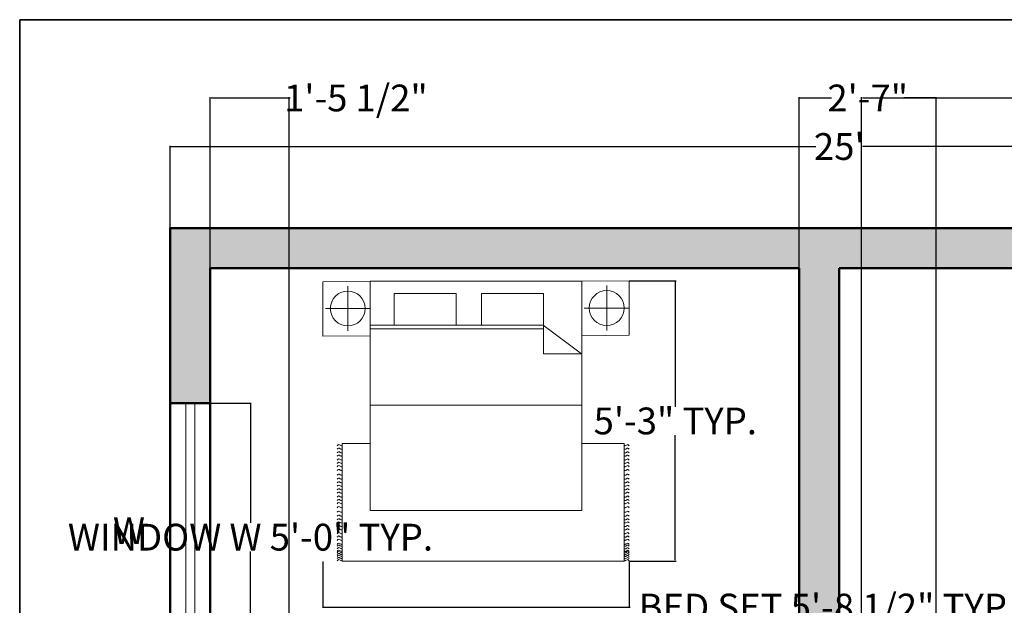
# Model space of a CAD drawing. Units: inches. Extents: x 125920 to 126336, y 366134 to 366735.
# Tile 5 of 6: x 125933 to 126153, y 366604 to 366735. Entities that reach past the tile are written whole.
import ezdxf

# ---------------------------------------------------------------- set-up
doc = ezdxf.new("R2010")
doc.units = ezdxf.units.IN
doc.header["$MEASUREMENT"] = 0
for name, color, linetype, lineweight in [('A-ANNO-DIMS', 2, 'Continuous', 18), ('A-ANNO-TEXT', 7, 'Continuous', 18), ('A-ANNO-TTLB', 7, 'Continuous', 35), ('A-FURN', 8, 'Continuous', 18), ('A-GLAZ', 4, 'Continuous', 18), ('A-WALL', 7, 'Continuous', 50)]:
    doc.layers.add(name, color=color, linetype=linetype, lineweight=lineweight)
doc.layers.add('A-WALL-PATT', color=18, linetype='Continuous', lineweight=13, true_color=0x000000)
doc.styles.get("Standard").update_dxf_attribs({"font": 'arial.ttf'})
doc.dimstyles.get("Standard").update_dxf_attribs({"dimtxt": 6, "dimasz": 0.18, "dimexe": 0.18, "dimexo": 0.0625, "dimgap": 0.09, "dimtad": 0, "dimtih": 1, "dimtoh": 1, "dimdec": 1, "dimzin": 0, "dimdsep": 46, "dimlunit": 3, "dimtxsty": 'Standard', "dimcen": 0.09, "dimadec": 0, "dimazin": 0, "dimtfac": 1, "dimtdec": 1, "dimtofl": 0, "dimtmove": 0, "dimatfit": 3, "dimfxl": 1, "dimtolj": 1, "dimtzin": 0, "dimarcsym": 0})

# ---------------------------------------------------------------- blocks, each defined once
blk = doc.blocks.new('*D3')
at = {"layer": 'A-ANNO-DIMS', "color": 0, "lineweight": -2, "transparency": 16777216}
for p, q in [((125966.47, 366688.86), (125966.47, 366707.25)), ((125966.65, 366707.07), (126111.24, 366707.07)), ((126266.29, 366707.07), (126121.71, 366707.07)), ((126266.47, 366688.86), (126266.47, 366707.25))]:
    blk.add_line(p, q, dxfattribs=at)
at = {"layer": 'A-ANNO-DIMS', "color": 0, "transparency": 16777216}
for points in [[(125966.65, 366707.1), (125966.65, 366707.04), (125966.47, 366707.07)], [(126266.29, 366707.1), (126266.29, 366707.04), (126266.47, 366707.07)]]:
    blk.add_solid(points, dxfattribs=at)
at = {"layer": 'Defpoints', "color": 0, "transparency": 16777216}
for p in [(126266.47, 366707.07), (125966.47, 366688.79), (126266.47, 366688.79)]:
    blk.add_point(p, dxfattribs=at)
at = {"layer": 'A-ANNO-DIMS', "color": 0, "transparency": 16777216, "insert": (126116.47, 366707.07), "char_height": 6, "attachment_point": 5}
blk.add_mtext("\\A1;25'", dxfattribs=at)
blk = doc.blocks.new('BED-DOUBLE-WITH-NIGHTSTANDS')
for p, q in [((5.6, 61.62), (5.6, 51.56)), ((63.65, 61.72), (63.65, 51.66)), ((10.63, 56.59), (0.57, 56.59)), ((68.68, 56.69), (58.62, 56.69)), ((49.39, 52.82), (10.63, 52.82)), ((49.44, 52), (10.63, 52)), ((49.39, 52.82), (58, 46.47)), ((49.44, 52.82), (49.44, 46.47)), ((49.44, 46.47), (58, 46.47)), ((58.05, 34.96), (10.63, 34.96)), ((4.36, 0), (4.36, 26.37)), ((4.36, 26.37), (10.65, 26.37)), ((58.05, 26.37), (67.59, 26.37)), ((67.59, 26.37), (67.59, 0)), ((67.59, 0), (4.36, 0))]:
    blk.add_line(p, q)
for points in [[(0, 50.39), (10.63, 50.5), (10.63, 62.68), (0, 62.58)], [(58.05, 62.68), (58.05, 11.37), (10.63, 11.37), (10.63, 62.68)], [(58.05, 50.5), (68.68, 50.6), (68.68, 62.78), (58.05, 62.68)], [(29.88, 59.98), (29.88, 52.82), (15.98, 52.82), (15.98, 59.98)], [(49.44, 59.98), (49.44, 52.82), (35.55, 52.82), (35.55, 59.98)]]:
    blk.add_lwpolyline(points, close=True)
for centre in [(5.6, 56.59), (63.65, 56.69)]:
    blk.add_circle(centre, 3.92)
for points, knots in [([(3.23, 25.84), (3.32, 25.96), (3.52, 26.2), (3.86, 25.96), (4.14, 25.78), (4.29, 25.89), (4.36, 25.94)], [0, 0, 0, 0, 0.400747, 0.791423, 1.067667, 1.29709, 1.29709, 1.29709, 1.29709]), ([(3.23, 25.06), (3.32, 25.18), (3.52, 25.42), (3.86, 25.18), (4.14, 25.01), (4.29, 25.11), (4.36, 25.16)], [0, 0, 0, 0, 0.400747, 0.791423, 1.067667, 1.29709, 1.29709, 1.29709, 1.29709]), ([(3.23, 24.24), (3.32, 24.36), (3.52, 24.6), (3.86, 24.36), (4.14, 24.19), (4.29, 24.3), (4.36, 24.34)], [0, 0, 0, 0, 0.400747, 0.791423, 1.067667, 1.29709, 1.29709, 1.29709, 1.29709]), ([(68.71, 25.84), (68.61, 25.96), (68.42, 26.2), (68.08, 25.96), (67.8, 25.78), (67.65, 25.89), (67.58, 25.94)], [0, 0, 0, 0, 0.400747, 0.791423, 1.067667, 1.29709, 1.29709, 1.29709, 1.29709]), ([(68.71, 25.06), (68.61, 25.18), (68.42, 25.42), (68.08, 25.18), (67.8, 25.01), (67.65, 25.11), (67.58, 25.16)], [0, 0, 0, 0, 0.400747, 0.791423, 1.067667, 1.29709, 1.29709, 1.29709, 1.29709]), ([(68.71, 24.24), (68.61, 24.36), (68.42, 24.6), (68.08, 24.36), (67.8, 24.19), (67.65, 24.3), (67.58, 24.34)], [0, 0, 0, 0, 0.400747, 0.791423, 1.067667, 1.29709, 1.29709, 1.29709, 1.29709]), ([(3.23, 23.51), (3.32, 23.63), (3.52, 23.87), (3.86, 23.63), (4.14, 23.46), (4.29, 23.57), (4.36, 23.62)], [0, 0, 0, 0, 0.400747, 0.791423, 1.067667, 1.29709, 1.29709, 1.29709, 1.29709]), ([(3.23, 22.63), (3.32, 22.75), (3.52, 22.99), (3.86, 22.75), (4.14, 22.58), (4.29, 22.69), (4.36, 22.73)], [0, 0, 0, 0, 0.400747, 0.791423, 1.067667, 1.29709, 1.29709, 1.29709, 1.29709]), ([(3.23, 21.88), (3.32, 22), (3.52, 22.24), (3.86, 22), (4.14, 21.83), (4.29, 21.93), (4.36, 21.98)], [0, 0, 0, 0, 0.400747, 0.791423, 1.067667, 1.29709, 1.29709, 1.29709, 1.29709]), ([(68.71, 23.51), (68.61, 23.63), (68.42, 23.87), (68.08, 23.63), (67.8, 23.46), (67.65, 23.57), (67.58, 23.62)], [0, 0, 0, 0, 0.400747, 0.791423, 1.067667, 1.29709, 1.29709, 1.29709, 1.29709]), ([(68.71, 22.63), (68.61, 22.75), (68.42, 22.99), (68.08, 22.75), (67.8, 22.58), (67.65, 22.69), (67.58, 22.73)], [0, 0, 0, 0, 0.400747, 0.791423, 1.067667, 1.29709, 1.29709, 1.29709, 1.29709]), ([(68.71, 21.88), (68.61, 22), (68.42, 22.24), (68.08, 22), (67.8, 21.83), (67.65, 21.93), (67.58, 21.98)], [0, 0, 0, 0, 0.400747, 0.791423, 1.067667, 1.29709, 1.29709, 1.29709, 1.29709]), ([(3.23, 21.15), (3.32, 21.27), (3.52, 21.51), (3.86, 21.27), (4.14, 21.1), (4.29, 21.21), (4.36, 21.25)], [0, 0, 0, 0, 0.400747, 0.791423, 1.067667, 1.29709, 1.29709, 1.29709, 1.29709]), ([(3.23, 20.27), (3.32, 20.39), (3.52, 20.63), (3.86, 20.39), (4.14, 20.22), (4.29, 20.32), (4.36, 20.37)], [0, 0, 0, 0, 0.400747, 0.791423, 1.067667, 1.29709, 1.29709, 1.29709, 1.29709]), ([(68.71, 21.15), (68.61, 21.27), (68.42, 21.51), (68.08, 21.27), (67.8, 21.1), (67.65, 21.21), (67.58, 21.25)], [0, 0, 0, 0, 0.400747, 0.791423, 1.067667, 1.29709, 1.29709, 1.29709, 1.29709]), ([(68.71, 20.27), (68.61, 20.39), (68.42, 20.63), (68.08, 20.39), (67.8, 20.22), (67.65, 20.32), (67.58, 20.37)], [0, 0, 0, 0, 0.400747, 0.791423, 1.067667, 1.29709, 1.29709, 1.29709, 1.29709]), ([(3.23, 19.23), (3.32, 19.35), (3.52, 19.59), (3.86, 19.35), (4.14, 19.18), (4.29, 19.29), (4.36, 19.33)], [0, 0, 0, 0, 0.400747, 0.791423, 1.067667, 1.29709, 1.29709, 1.29709, 1.29709]), ([(3.23, 18.35), (3.32, 18.47), (3.52, 18.71), (3.86, 18.47), (4.14, 18.3), (4.29, 18.4), (4.36, 18.45)], [0, 0, 0, 0, 0.400747, 0.791423, 1.067667, 1.29709, 1.29709, 1.29709, 1.29709]), ([(3.23, 17.53), (3.32, 17.65), (3.52, 17.89), (3.86, 17.65), (4.14, 17.48), (4.29, 17.59), (4.36, 17.64)], [0, 0, 0, 0, 0.400747, 0.791423, 1.067667, 1.29709, 1.29709, 1.29709, 1.29709]), ([(68.71, 19.23), (68.61, 19.35), (68.42, 19.59), (68.08, 19.35), (67.8, 19.18), (67.65, 19.29), (67.58, 19.33)], [0, 0, 0, 0, 0.400747, 0.791423, 1.067667, 1.29709, 1.29709, 1.29709, 1.29709]), ([(68.71, 18.35), (68.61, 18.47), (68.42, 18.71), (68.08, 18.47), (67.8, 18.3), (67.65, 18.4), (67.58, 18.45)], [0, 0, 0, 0, 0.400747, 0.791423, 1.067667, 1.29709, 1.29709, 1.29709, 1.29709]), ([(68.71, 17.53), (68.61, 17.65), (68.42, 17.89), (68.08, 17.65), (67.8, 17.48), (67.65, 17.59), (67.58, 17.64)], [0, 0, 0, 0, 0.400747, 0.791423, 1.067667, 1.29709, 1.29709, 1.29709, 1.29709]), ([(3.23, 16.76), (3.32, 16.88), (3.52, 17.12), (3.86, 16.88), (4.14, 16.7), (4.29, 16.81), (4.36, 16.86)], [0, 0, 0, 0, 0.400747, 0.791423, 1.067667, 1.29709, 1.29709, 1.29709, 1.29709]), ([(3.23, 15.94), (3.32, 16.06), (3.52, 16.3), (3.86, 16.06), (4.14, 15.89), (4.29, 16), (4.36, 16.04)], [0, 0, 0, 0, 0.400747, 0.791423, 1.067667, 1.29709, 1.29709, 1.29709, 1.29709]), ([(3.23, 15.21), (3.32, 15.33), (3.52, 15.57), (3.86, 15.33), (4.14, 15.16), (4.29, 15.27), (4.36, 15.32)], [0, 0, 0, 0, 0.400747, 0.791423, 1.067667, 1.29709, 1.29709, 1.29709, 1.29709]), ([(68.71, 16.76), (68.61, 16.88), (68.42, 17.12), (68.08, 16.88), (67.8, 16.7), (67.65, 16.81), (67.58, 16.86)], [0, 0, 0, 0, 0.400747, 0.791423, 1.067667, 1.29709, 1.29709, 1.29709, 1.29709]), ([(68.71, 15.94), (68.61, 16.06), (68.42, 16.3), (68.08, 16.06), (67.8, 15.89), (67.65, 16), (67.58, 16.04)], [0, 0, 0, 0, 0.400747, 0.791423, 1.067667, 1.29709, 1.29709, 1.29709, 1.29709]), ([(68.71, 15.21), (68.61, 15.33), (68.42, 15.57), (68.08, 15.33), (67.8, 15.16), (67.65, 15.27), (67.58, 15.32)], [0, 0, 0, 0, 0.400747, 0.791423, 1.067667, 1.29709, 1.29709, 1.29709, 1.29709]), ([(3.23, 14.33), (3.32, 14.45), (3.52, 14.69), (3.86, 14.45), (4.14, 14.28), (4.29, 14.38), (4.36, 14.43)], [0, 0, 0, 0, 0.400747, 0.791423, 1.067667, 1.29709, 1.29709, 1.29709, 1.29709]), ([(3.23, 13.58), (3.32, 13.7), (3.52, 13.94), (3.86, 13.7), (4.14, 13.53), (4.29, 13.63), (4.36, 13.68)], [0, 0, 0, 0, 0.400747, 0.791423, 1.067667, 1.29709, 1.29709, 1.29709, 1.29709]), ([(68.71, 14.33), (68.61, 14.45), (68.42, 14.69), (68.08, 14.45), (67.8, 14.28), (67.65, 14.38), (67.58, 14.43)], [0, 0, 0, 0, 0.400747, 0.791423, 1.067667, 1.29709, 1.29709, 1.29709, 1.29709]), ([(68.71, 13.58), (68.61, 13.7), (68.42, 13.94), (68.08, 13.7), (67.8, 13.53), (67.65, 13.63), (67.58, 13.68)], [0, 0, 0, 0, 0.400747, 0.791423, 1.067667, 1.29709, 1.29709, 1.29709, 1.29709]), ([(3.23, 12.85), (3.32, 12.97), (3.52, 13.21), (3.86, 12.97), (4.14, 12.8), (4.29, 12.9), (4.36, 12.95)], [0, 0, 0, 0, 0.400747, 0.791423, 1.067667, 1.29709, 1.29709, 1.29709, 1.29709]), ([(3.23, 11.97), (3.32, 12.09), (3.52, 12.33), (3.86, 12.09), (4.14, 11.92), (4.29, 12.02), (4.36, 12.07)], [0, 0, 0, 0, 0.400747, 0.791423, 1.067667, 1.29709, 1.29709, 1.29709, 1.29709]), ([(3.23, 10.93), (3.32, 11.05), (3.52, 11.29), (3.86, 11.05), (4.14, 10.88), (4.29, 10.99), (4.36, 11.03)], [0, 0, 0, 0, 0.400747, 0.791423, 1.067667, 1.29709, 1.29709, 1.29709, 1.29709]), ([(68.71, 12.85), (68.61, 12.97), (68.42, 13.21), (68.08, 12.97), (67.8, 12.8), (67.65, 12.9), (67.58, 12.95)], [0, 0, 0, 0, 0.400747, 0.791423, 1.067667, 1.29709, 1.29709, 1.29709, 1.29709]), ([(68.71, 11.97), (68.61, 12.09), (68.42, 12.33), (68.08, 12.09), (67.8, 11.92), (67.65, 12.02), (67.58, 12.07)], [0, 0, 0, 0, 0.400747, 0.791423, 1.067667, 1.29709, 1.29709, 1.29709, 1.29709]), ([(68.71, 10.93), (68.61, 11.05), (68.42, 11.29), (68.08, 11.05), (67.8, 10.88), (67.65, 10.99), (67.58, 11.03)], [0, 0, 0, 0, 0.400747, 0.791423, 1.067667, 1.29709, 1.29709, 1.29709, 1.29709]), ([(3.23, 10.05), (3.32, 10.17), (3.52, 10.41), (3.86, 10.17), (4.14, 10), (4.29, 10.1), (4.36, 10.15)], [0, 0, 0, 0, 0.400747, 0.791423, 1.067667, 1.29709, 1.29709, 1.29709, 1.29709]), ([(3.23, 9.23), (3.32, 9.35), (3.52, 9.59), (3.86, 9.35), (4.14, 9.18), (4.29, 9.29), (4.36, 9.34)], [0, 0, 0, 0, 0.400747, 0.791423, 1.067667, 1.29709, 1.29709, 1.29709, 1.29709]), ([(68.71, 10.05), (68.61, 10.17), (68.42, 10.41), (68.08, 10.17), (67.8, 10), (67.65, 10.1), (67.58, 10.15)], [0, 0, 0, 0, 0.400747, 0.791423, 1.067667, 1.29709, 1.29709, 1.29709, 1.29709]), ([(68.71, 9.23), (68.61, 9.35), (68.42, 9.59), (68.08, 9.35), (67.8, 9.18), (67.65, 9.29), (67.58, 9.34)], [0, 0, 0, 0, 0.400747, 0.791423, 1.067667, 1.29709, 1.29709, 1.29709, 1.29709]), ([(3.23, 8.54), (3.32, 8.66), (3.52, 8.9), (3.86, 8.66), (4.14, 8.49), (4.29, 8.6), (4.36, 8.65)], [0, 0, 0, 0, 0.400747, 0.791423, 1.067667, 1.29709, 1.29709, 1.29709, 1.29709]), ([(3.23, 7.73), (3.32, 7.85), (3.52, 8.09), (3.86, 7.85), (4.14, 7.68), (4.29, 7.78), (4.36, 7.83)], [0, 0, 0, 0, 0.400747, 0.791423, 1.067667, 1.29709, 1.29709, 1.29709, 1.29709]), ([(3.23, 7), (3.32, 7.12), (3.52, 7.36), (3.86, 7.12), (4.14, 6.95), (4.29, 7.05), (4.36, 7.1)], [0, 0, 0, 0, 0.400747, 0.791423, 1.067667, 1.29709, 1.29709, 1.29709, 1.29709]), ([(68.71, 8.54), (68.61, 8.66), (68.42, 8.9), (68.08, 8.66), (67.8, 8.49), (67.65, 8.6), (67.58, 8.65)], [0, 0, 0, 0, 0.400747, 0.791423, 1.067667, 1.29709, 1.29709, 1.29709, 1.29709]), ([(68.71, 7.73), (68.61, 7.85), (68.42, 8.09), (68.08, 7.85), (67.8, 7.68), (67.65, 7.78), (67.58, 7.83)], [0, 0, 0, 0, 0.400747, 0.791423, 1.067667, 1.29709, 1.29709, 1.29709, 1.29709]), ([(68.71, 7), (68.61, 7.12), (68.42, 7.36), (68.08, 7.12), (67.8, 6.95), (67.65, 7.05), (67.58, 7.1)], [0, 0, 0, 0, 0.400747, 0.791423, 1.067667, 1.29709, 1.29709, 1.29709, 1.29709]), ([(3.23, 6.12), (3.32, 6.24), (3.52, 6.48), (3.86, 6.24), (4.14, 6.07), (4.29, 6.17), (4.36, 6.22)], [0, 0, 0, 0, 0.400747, 0.791423, 1.067667, 1.29709, 1.29709, 1.29709, 1.29709]), ([(3.23, 5.36), (3.32, 5.49), (3.52, 5.73), (3.86, 5.49), (4.14, 5.31), (4.29, 5.42), (4.36, 5.47)], [0, 0, 0, 0, 0.400747, 0.791423, 1.067667, 1.29709, 1.29709, 1.29709, 1.29709]), ([(3.23, 4.64), (3.32, 4.76), (3.52, 5), (3.86, 4.76), (4.14, 4.59), (4.29, 4.69), (4.36, 4.74)], [0, 0, 0, 0, 0.400747, 0.791423, 1.067667, 1.29709, 1.29709, 1.29709, 1.29709]), ([(68.71, 6.12), (68.61, 6.24), (68.42, 6.48), (68.08, 6.24), (67.8, 6.07), (67.65, 6.17), (67.58, 6.22)], [0, 0, 0, 0, 0.400747, 0.791423, 1.067667, 1.29709, 1.29709, 1.29709, 1.29709]), ([(68.71, 5.36), (68.61, 5.49), (68.42, 5.73), (68.08, 5.49), (67.8, 5.31), (67.65, 5.42), (67.58, 5.47)], [0, 0, 0, 0, 0.400747, 0.791423, 1.067667, 1.29709, 1.29709, 1.29709, 1.29709]), ([(68.71, 4.64), (68.61, 4.76), (68.42, 5), (68.08, 4.76), (67.8, 4.59), (67.66, 4.69), (67.59, 4.73)], [0, 0, 0, 0, 0.400747, 0.791423, 1.067667, 1.283686, 1.283686, 1.283686, 1.283686]), ([(3.23, 3.75), (3.32, 3.88), (3.52, 4.12), (3.86, 3.88), (4.14, 3.7), (4.29, 3.81), (4.36, 3.86)], [0, 0, 0, 0, 0.400747, 0.791423, 1.067667, 1.29709, 1.29709, 1.29709, 1.29709]), ([(3.23, 3.33), (3.32, 3.45), (3.52, 3.7), (3.86, 3.44), (4.14, 3.27), (4.29, 3.38), (4.36, 3.43)], [0, 0, 0, 0, 0.407265, 0.802015, 1.07826, 1.307683, 1.307683, 1.307683, 1.307683]), ([(3.23, 2.76), (3.32, 2.88), (3.52, 3.12), (3.86, 2.88), (4.14, 2.71), (4.29, 2.81), (4.36, 2.86)], [0, 0, 0, 0, 0.400747, 0.791423, 1.067667, 1.29709, 1.29709, 1.29709, 1.29709]), ([(3.23, 2.18), (3.32, 2.31), (3.52, 2.55), (3.86, 2.31), (4.14, 2.13), (4.29, 2.24), (4.36, 2.29)], [0, 0, 0, 0, 0.400747, 0.791423, 1.067667, 1.29709, 1.29709, 1.29709, 1.29709]), ([(68.71, 3.75), (68.61, 3.88), (68.42, 4.11), (68.08, 3.88), (67.8, 3.7), (67.66, 3.81), (67.59, 3.85)], [0, 0, 0, 0, 0.400747, 0.791423, 1.067667, 1.283686, 1.283686, 1.283686, 1.283686]), ([(68.71, 3.33), (68.61, 3.45), (68.42, 3.69), (68.08, 3.45), (67.8, 3.27), (67.66, 3.38), (67.59, 3.42)], [0, 0, 0, 0, 0.402903, 0.794912, 1.071156, 1.287177, 1.287177, 1.287177, 1.287177]), ([(68.71, 2.73), (68.61, 2.85), (68.42, 3.09), (68.08, 2.85), (67.8, 2.68), (67.66, 2.78), (67.59, 2.82)], [0, 0, 0, 0, 0.400747, 0.791423, 1.067667, 1.283686, 1.283686, 1.283686, 1.283686]), ([(68.71, 2.16), (68.61, 2.28), (68.42, 2.52), (68.08, 2.28), (67.8, 2.11), (67.66, 2.21), (67.59, 2.25)], [0, 0, 0, 0, 0.400747, 0.791423, 1.067667, 1.283686, 1.283686, 1.283686, 1.283686]), ([(3.23, 1.88), (3.32, 2), (3.52, 2.24), (3.86, 2), (4.14, 1.82), (4.29, 1.93), (4.36, 1.98)], [0, 0, 0, 0, 0.400747, 0.791423, 1.067667, 1.29709, 1.29709, 1.29709, 1.29709]), ([(3.23, 1.46), (3.32, 1.58), (3.52, 1.82), (3.86, 1.58), (4.14, 1.41), (4.29, 1.51), (4.36, 1.56)], [0, 0, 0, 0, 0.400747, 0.791423, 1.067667, 1.29709, 1.29709, 1.29709, 1.29709]), ([(3.23, 1.06), (3.32, 1.18), (3.52, 1.42), (3.86, 1.18), (4.14, 1.01), (4.29, 1.11), (4.36, 1.16)], [0, 0, 0, 0, 0.400747, 0.791423, 1.067667, 1.29709, 1.29709, 1.29709, 1.29709]), ([(3.23, 0.57), (3.32, 0.7), (3.52, 0.94), (3.86, 0.7), (4.14, 0.52), (4.29, 0.63), (4.36, 0.68)], [0, 0, 0, 0, 0.400747, 0.791423, 1.067667, 1.29709, 1.29709, 1.29709, 1.29709]), ([(3.23, 0.07), (3.32, 0.19), (3.52, 0.43), (3.86, 0.19), (4.14, 0.02), (4.29, 0.13), (4.36, 0.18)], [0, 0, 0, 0, 0.400747, 0.791423, 1.067667, 1.29709, 1.29709, 1.29709, 1.29709]), ([(68.71, 1.43), (68.61, 1.55), (68.42, 1.79), (68.08, 1.55), (67.8, 1.38), (67.65, 1.48), (67.58, 1.53)], [0, 0, 0, 0, 0.400747, 0.791423, 1.067667, 1.29709, 1.29709, 1.29709, 1.29709]), ([(68.71, 1.03), (68.61, 1.15), (68.42, 1.39), (68.08, 1.15), (67.8, 0.98), (67.65, 1.09), (67.58, 1.13)], [0, 0, 0, 0, 0.400747, 0.791423, 1.067667, 1.29709, 1.29709, 1.29709, 1.29709]), ([(68.71, 0.55), (68.61, 0.67), (68.42, 0.91), (68.08, 0.67), (67.8, 0.49), (67.65, 0.6), (67.58, 0.65)], [0, 0, 0, 0, 0.400747, 0.791423, 1.067667, 1.29709, 1.29709, 1.29709, 1.29709]), ([(68.71, 0.07), (68.61, 0.19), (68.42, 0.43), (68.08, 0.19), (67.8, 0.02), (67.65, 0.13), (67.58, 0.18)], [0, 0, 0, 0, 0.400747, 0.791423, 1.067667, 1.29709, 1.29709, 1.29709, 1.29709]), ([(68.71, 1.85), (68.61, 1.97), (68.42, 2.21), (68.08, 1.97), (67.8, 1.8), (67.66, 1.9), (67.59, 1.94)], [0, 0, 0, 0, 0.400747, 0.791423, 1.067667, 1.283686, 1.283686, 1.283686, 1.283686])]:
    blk.add_open_spline(points, degree=3, knots=knots)
blk = doc.blocks.new('WIN-60')
for p, q in [((0, 0), (0, 60)), ((3.5, 0), (3.5, 60)), ((5.5, 60), (5.5, 0)), ((9, 60), (9, 0))]:
    blk.add_line(p, q)
blk = doc.blocks.new('*D13')
at = {"layer": 'A-ANNO-DIMS', "color": 0, "lineweight": -2, "transparency": 16777216}
for p, q in [((125975.54, 366649.55), (125984.65, 366649.55)), ((125984.47, 366649.37), (125984.47, 366622.75)), ((125984.47, 366589.73), (125984.47, 366616.36)), ((125975.54, 366589.55), (125984.65, 366589.55))]:
    blk.add_line(p, q, dxfattribs=at)
at = {"layer": 'A-ANNO-DIMS', "color": 0, "transparency": 16777216}
for points in [[(125984.44, 366649.37), (125984.5, 366649.37), (125984.47, 366649.55)], [(125984.44, 366589.73), (125984.5, 366589.73), (125984.47, 366589.55)]]:
    blk.add_solid(points, dxfattribs=at)
at = {"layer": 'Defpoints', "color": 0, "transparency": 16777216}
for p in [(125975.47, 366649.55), (125984.47, 366649.55), (125975.47, 366589.55)]:
    blk.add_point(p, dxfattribs=at)
at = {"layer": 'A-ANNO-DIMS', "color": 0, "transparency": 16777216, "insert": (125984.47, 366619.55), "char_height": 6, "attachment_point": 5}
blk.add_mtext('\\A1;WINDOW W 5\'-0" TYP.', dxfattribs=at)
blk = doc.blocks.new('*D19')
at = {"layer": 'A-ANNO-DIMS', "color": 0, "lineweight": -2, "transparency": 16777216}
for p, q in [((126000.69, 366614.13), (126000.69, 366603.71)), ((126069.4, 366614.13), (126069.4, 366603.71)), ((126000.87, 366603.89), (126069.22, 366603.89)), ((126069.4, 366603.89), (126069.58, 366603.89))]:
    blk.add_line(p, q, dxfattribs=at)
at = {"layer": 'A-ANNO-DIMS', "color": 0, "transparency": 16777216}
for points in [[(126000.87, 366603.92), (126000.87, 366603.86), (126000.69, 366603.89)], [(126069.22, 366603.92), (126069.22, 366603.86), (126069.4, 366603.89)]]:
    blk.add_solid(points, dxfattribs=at)
at = {"layer": 'Defpoints', "color": 0, "transparency": 16777216}
for p in [(126000.69, 366614.19), (126069.4, 366614.19), (126069.4, 366603.89)]:
    blk.add_point(p, dxfattribs=at)
at = {"layer": 'A-ANNO-DIMS', "color": 0, "transparency": 16777216, "insert": (126113.91, 366603.89), "char_height": 6, "attachment_point": 5}
blk.add_mtext('\\A1;BED SET 5\'-8 1/2" TYP.', dxfattribs=at)
blk = doc.blocks.new('*D20')
at = {"layer": 'A-ANNO-DIMS', "color": 0, "lineweight": -2, "transparency": 16777216}
for p, q in [((126069.46, 366676.98), (126079.89, 366676.98)), ((126079.71, 366676.8), (126079.71, 366648.74)), ((126079.71, 366614.37), (126079.71, 366642.43)), ((126069.46, 366614.19), (126079.89, 366614.19))]:
    blk.add_line(p, q, dxfattribs=at)
at = {"layer": 'A-ANNO-DIMS', "color": 0, "transparency": 16777216}
for points in [[(126079.68, 366676.8), (126079.74, 366676.8), (126079.71, 366676.98)], [(126079.68, 366614.37), (126079.74, 366614.37), (126079.71, 366614.19)]]:
    blk.add_solid(points, dxfattribs=at)
at = {"layer": 'Defpoints', "color": 0, "transparency": 16777216}
for p in [(126069.4, 366676.98), (126079.71, 366676.98), (126069.4, 366614.19)]:
    blk.add_point(p, dxfattribs=at)
at = {"layer": 'A-ANNO-DIMS', "color": 0, "transparency": 16777216, "insert": (126079.71, 366645.59), "char_height": 6, "attachment_point": 5}
blk.add_mtext('\\A1;5\'-3" TYP.', dxfattribs=at)
blk = doc.blocks.new('*D40')
at = {"layer": 'A-ANNO-DIMS', "color": 0, "lineweight": -2, "transparency": 16777216}
for p, q in [((126107.47, 366288.86), (126107.47, 366718.12)), ((126107.65, 366717.94), (126114.73, 366717.94)), ((126138.05, 366717.94), (126130.97, 366717.94)), ((126138.23, 366288.86), (126138.23, 366718.12))]:
    blk.add_line(p, q, dxfattribs=at)
at = {"layer": 'A-ANNO-DIMS', "color": 0, "transparency": 16777216}
for points in [[(126107.65, 366717.97), (126107.65, 366717.91), (126107.47, 366717.94)], [(126138.05, 366717.97), (126138.05, 366717.91), (126138.23, 366717.94)]]:
    blk.add_solid(points, dxfattribs=at)
at = {"layer": 'Defpoints', "color": 0, "transparency": 16777216}
for p in [(126138.23, 366717.94), (126107.47, 366288.79), (126138.23, 366288.79)]:
    blk.add_point(p, dxfattribs=at)
at = {"layer": 'A-ANNO-DIMS', "color": 0, "transparency": 16777216, "insert": (126122.85, 366717.94), "char_height": 6, "attachment_point": 5}
blk.add_mtext('\\A1;2\'-7"', dxfattribs=at)
blk = doc.blocks.new('*D41')
at = {"layer": 'A-ANNO-DIMS', "color": 0, "lineweight": -2, "transparency": 16777216}
for p, q in [((126121.47, 366216.86), (126121.47, 366718.12)), ((126121.65, 366717.94), (126163.4, 366717.94)), ((126221.29, 366717.94), (126179.54, 366717.94)), ((126221.47, 366216.86), (126221.47, 366718.12))]:
    blk.add_line(p, q, dxfattribs=at)
at = {"layer": 'A-ANNO-DIMS', "color": 0, "transparency": 16777216}
for points in [[(126121.65, 366717.97), (126121.65, 366717.91), (126121.47, 366717.94)], [(126221.29, 366717.97), (126221.29, 366717.91), (126221.47, 366717.94)]]:
    blk.add_solid(points, dxfattribs=at)
at = {"layer": 'Defpoints', "color": 0, "transparency": 16777216}
for p in [(126221.47, 366717.94), (126121.47, 366216.79), (126221.47, 366216.79)]:
    blk.add_point(p, dxfattribs=at)
at = {"layer": 'A-ANNO-DIMS', "color": 0, "transparency": 16777216, "insert": (126171.47, 366717.94), "char_height": 6, "attachment_point": 5}
blk.add_mtext('\\A1;8\'-4"', dxfattribs=at)
blk = doc.blocks.new('*D45')
at = {"layer": 'A-ANNO-DIMS', "color": 0, "lineweight": -2, "transparency": 16777216}
for p, q in [((125975.47, 366216.86), (125975.47, 366718.12)), ((125975.65, 366717.94), (125992.98, 366717.94)), ((125993.16, 366235.36), (125993.16, 366718.12)), ((125993.16, 366717.94), (125993.34, 366717.94))]:
    blk.add_line(p, q, dxfattribs=at)
at = {"layer": 'A-ANNO-DIMS', "color": 0, "transparency": 16777216}
for points in [[(125975.65, 366717.97), (125975.65, 366717.91), (125975.47, 366717.94)], [(125992.98, 366717.97), (125992.98, 366717.91), (125993.16, 366717.94)]]:
    blk.add_solid(points, dxfattribs=at)
at = {"layer": 'Defpoints', "color": 0, "transparency": 16777216}
for p in [(125993.16, 366717.94), (125993.16, 366235.3), (125975.47, 366216.79)]:
    blk.add_point(p, dxfattribs=at)
at = {"layer": 'A-ANNO-DIMS', "color": 0, "transparency": 16777216, "insert": (126008.11, 366717.94), "char_height": 6, "attachment_point": 5}
blk.add_mtext('\\A1;1\'-5 1/2"', dxfattribs=at)

msp = doc.modelspace()

# ---------------------------------------------------------------- hatches: boundary and pattern name
at = {"layer": 'A-WALL-PATT'}
h = msp.add_hatch(color=256, dxfattribs=at)
h.dxf.hatch_style = 1
h.paths.add_polyline_path([(126266.47, 366688.79), (125966.47, 366688.79), (125966.47, 366649.55), (125975.47, 366649.55), (125975.47, 366679.79), (126107.47, 366679.79), (126107.47, 366547.79), (126106.47, 366547.79), (126106.47, 366538.79), (126107.47, 366538.79), (126117.47, 366538.79), (126117.47, 366547.79), (126116.47, 366547.79), (126116.47, 366679.79), (126257.47, 366679.79), (126257.47, 366648.33), (126266.47, 366648.33)])
h.paths.add_polyline_path([(126070.47, 366547.79), (125975.47, 366547.79), (125975.47, 366589.55), (125966.47, 366589.55), (125966.47, 366528.42), (125975.47, 366528.42), (125975.47, 366538.79), (126059.47, 366538.79), (126059.47, 366515.79), (126063.97, 366515.79), (126063.97, 366538.79), (126070.47, 366538.79)])
h.paths.add_polyline_path([(125975.47, 366486.29), (126063.97, 366486.29), (126063.97, 366491.79), (126059.47, 366491.79), (126059.47, 366490.79), (125975.47, 366490.79), (125975.47, 366504.42), (125966.47, 366504.42), (125966.47, 366437.07), (125975.47, 366437.07)])
h.paths.add_polyline_path([(125975.47, 366312.79), (126022.47, 366312.79), (126022.47, 366317.29), (125975.47, 366317.29), (125975.47, 366377.07), (125966.47, 366377.07), (125966.47, 366207.79), (125987.64, 366207.79), (125987.64, 366216.79), (125975.47, 366216.79)])
h.paths.add_polyline_path([(126063.97, 366216.79), (126063.97, 366312.79), (126070.47, 366312.79), (126070.47, 366317.29), (126058.47, 366317.29), (126058.47, 366312.79), (126059.47, 366312.79), (126059.47, 366216.79), (126047.64, 366216.79), (126047.64, 366207.79), (126063.97, 366207.79)])
h.paths.add_polyline_path([(126221.47, 366216.79), (126116.47, 366216.79), (126107.47, 366216.79), (126107.47, 366207.79), (126221.47, 366207.79)])
h.paths.add_polyline_path([(126266.47, 366336.48), (126257.47, 366336.48), (126257.47, 366297.79), (126174.23, 366297.79), (126174.23, 366288.79), (126257.47, 366288.79), (126257.47, 366207.79), (126266.47, 366207.79)])
h.paths.add_polyline_path([(126138.23, 366297.79), (126116.47, 366297.79), (126116.47, 366433.79), (126117.47, 366433.79), (126117.47, 366438.29), (126116.47, 366438.29), (126107.47, 366438.29), (126107.47, 366317.29), (126106.47, 366317.29), (126106.47, 366312.79), (126107.47, 366312.79), (126107.47, 366288.79), (126116.47, 366288.79), (126138.23, 366288.79)])
h.paths.add_polyline_path([(126266.47, 366449.1), (126257.47, 366449.1), (126257.47, 366438.29), (126256.47, 366438.29), (126256.47, 366433.79), (126257.47, 366433.79), (126257.47, 366396.48), (126266.47, 366396.48)])
h.paths.add_polyline_path([(126232.47, 366438.29), (126180.47, 366438.29), (126180.47, 366486.29), (126257.47, 366486.29), (126257.47, 366473.1), (126266.47, 366473.1), (126266.47, 366504.78), (126257.47, 366504.78), (126257.47, 366490.79), (126180.47, 366490.79), (126180.47, 366538.79), (126232.47, 366538.79), (126232.47, 366547.79), (126153.47, 366547.79), (126153.47, 366538.79), (126175.97, 366538.79), (126175.97, 366438.29), (126153.47, 366438.29), (126153.47, 366433.79), (126232.47, 366433.79)])
h.paths.add_polyline_path([(126266.47, 366588.33), (126257.47, 366588.33), (126257.47, 366547.79), (126256.47, 366547.79), (126256.47, 366538.79), (126257.47, 366538.79), (126257.47, 366528.78), (126266.47, 366528.78)])

# ---------------------------------------------------------------- linework, layer by layer
at = {"layer": 'A-ANNO-TTLB'}
msp.add_lwpolyline([(125932.73, 366735.48), (126336.24, 366735.48), (126336.24, 366133.52), (125932.73, 366133.52)], close=True, dxfattribs=at)
at = {"layer": 'A-WALL'}
for p, q in [((125966.47, 366688.79), (126266.47, 366688.79)), ((125966.47, 366688.79), (125966.47, 366207.79)), ((125975.47, 366679.79), (125975.47, 366547.79)), ((125975.47, 366679.79), (126107.47, 366679.79)), ((126107.47, 366679.79), (126107.47, 366547.79)), ((126107.47, 366679.79), (126107.47, 366547.79)), ((126116.47, 366679.79), (126116.47, 366547.79)), ((126116.47, 366679.79), (126116.47, 366547.79)), ((126116.47, 366679.79), (126257.47, 366679.79)), ((125966.47, 366649.55), (125975.47, 366649.55))]:
    msp.add_line(p, q, dxfattribs=at)

# ---------------------------------------------------------------- block references
at = {"layer": 'A-FURN'}
msp.add_blockref('BED-DOUBLE-WITH-NIGHTSTANDS', (126000.69, 366614.19), dxfattribs=at)
at = {"layer": 'A-GLAZ'}
msp.add_blockref('WIN-60', (125966.47, 366589.55), dxfattribs=at)

# ---------------------------------------------------------------- texts
at = {"layer": 'A-ANNO-TEXT', "insert": (125953.64, 366624), "char_height": 6, "attachment_point": 1}
msp.add_mtext_dynamic_manual_height_columns('W', width=14.507, gutter_width=30, heights=[0], dxfattribs=at)

# ---------------------------------------------------------------- dimensions: what is measured, and where the dimension line sits
at = {"layer": 'A-ANNO-DIMS'}
for base, p1, p2, override, picture, middle in [((125993.16, 366717.94), (125975.47, 366216.79), (125993.16, 366235.3), {"dimdec": 1, "dimlfac": 1, "dimrnd": 0, "dimzin": 1, "dimdsep": 46, "dimlunit": 4, "dimfrac": 2}, '*D45', (126008.11, 366717.94)), ((126138.23, 366717.94), (126107.47, 366288.79), (126138.23, 366288.79), {"dimdec": 1, "dimlfac": 1, "dimrnd": 0, "dimzin": 1, "dimdsep": 46, "dimlunit": 4, "dimfrac": 2}, '*D40', (126122.85, 366717.94)), ((126221.47, 366717.94), (126121.47, 366216.79), (126221.47, 366216.79), {"dimdec": 1, "dimlfac": 1, "dimrnd": 0, "dimzin": 1, "dimdsep": 46, "dimlunit": 4, "dimfrac": 2}, '*D41', (126171.47, 366717.94)), ((126266.47, 366707.07), (125966.47, 366688.79), (126266.47, 366688.79), {"dimclrd": 0, "dimclre": 0, "dimclrt": 0}, '*D3', (126116.47, 366707.07))]:
    dim = msp.add_linear_dim(base=base, p1=p1, p2=p2, dimstyle='Standard', override=override, dxfattribs=at)
    dim.commit()
    dim.dimension.update_dxf_attribs({"geometry": picture, "text_midpoint": middle})
for base, p1, p2, text, picture, middle in [((126079.71, 366676.98), (126069.4, 366614.19), (126069.4, 366676.98), '<> TYP.', '*D20', (126079.71, 366645.59)), ((125984.47, 366649.55), (125975.47, 366589.55), (125975.47, 366649.55), 'WINDOW W <> TYP.', '*D13', (125984.47, 366619.55))]:
    dim = msp.add_linear_dim(base=base, p1=p1, p2=p2, angle=90, text=text, dimstyle='Standard', override={"dimdec": 1, "dimlfac": 1, "dimrnd": 0, "dimzin": 1, "dimdsep": 46, "dimlunit": 4, "dimfrac": 2}, dxfattribs=at)
    dim.commit()
    dim.dimension.update_dxf_attribs({"geometry": picture, "text_midpoint": middle})
dim = msp.add_linear_dim(base=(126069.4, 366603.89), p1=(126000.69, 366614.19), p2=(126069.4, 366614.19), text='BED SET <> TYP.', dimstyle='Standard', override={"dimdec": 1, "dimlfac": 1, "dimrnd": 0, "dimzin": 1, "dimdsep": 46, "dimlunit": 4, "dimfrac": 2}, dxfattribs=at)
dim.commit()
dim.dimension.update_dxf_attribs({"geometry": '*D19', "text_midpoint": (126113.91, 366603.89)})

doc.saveas('drawing.dxf')
